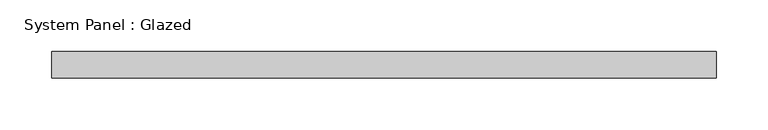
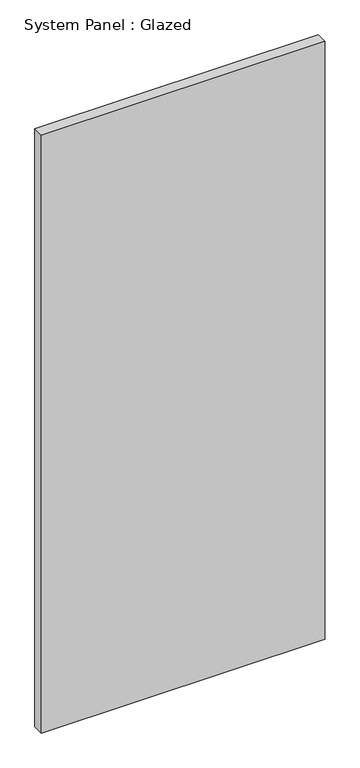
"""IFC4 building model written with IfcOpenShell, lengths in millimetres: plate geometry, System Panel : Glazed."""

from ifc_helpers import new_model, si_unit, origin, origin_with_axes, place, context, project, spatial, polyline, outline, extrude, source, transform, mapped, element, save


def system_panel_glazed_3037aa96(model_context):
    return source(origin(), model_context, "Body", "SweptSolid", [
        extrude(outline(polyline([(320.675, 19.05), (-320.675, 19.05), (-320.675, 44.45), (320.675, 44.45), (320.675, 19.05)])), origin_with_axes(), (0.0, 0.0, 1.0), 1430.357611),
    ])


if __name__ == "__main__":
    model = new_model("IFC4")
    model_context = context("Model", 3, world=origin())
    ifc_project = project(units=[si_unit("LENGTHUNIT", "METRE", prefix="MILLI")], contexts=[model_context])
    site = spatial("IfcSite", under=ifc_project)
    building = spatial("IfcBuilding", under=site)
    placement = place(None, origin())
    system_panel_glazed_shape = system_panel_glazed_3037aa96(model_context)
    element("IfcPlate", 1, ObjectType="System Panel : Glazed", at=placement, inside=building, context=model_context, shape_type="MappedRepresentation", body=[
        mapped(system_panel_glazed_shape, transform((0.0, 0.0, 0.0), x_axis=(1.0, 0.0, 0.0), y_axis=(0.0, 1.0, 0.0), z_axis=(0.0, 0.0, 1.0))),
    ])
    save(model, "model.ifc")

# Revit data of these elements
# Type "System Panel : Glazed"
#   Construction Type Id = "GSP4R"
#   Analytic Construction = "1/8 in Pilkington single glazing"
#   Visual Light Transmittance = 0.9
#   Solar Heat Gain Coefficient = 0.86
#   Heat Transfer Coefficient (U) = 1.18115 BTU/(h·ft²·°F)
#   Define Thermal Properties by = 1
# Element 1 (IfcPlate, "System Panel : Glazed")
#   Materials on its faces: "Glass"
# Materials
#   "Glass": class "Glass", colour RGB 0 128 192, transparency 0.75, Description = "Soda Lime Glass", Cost = 0
